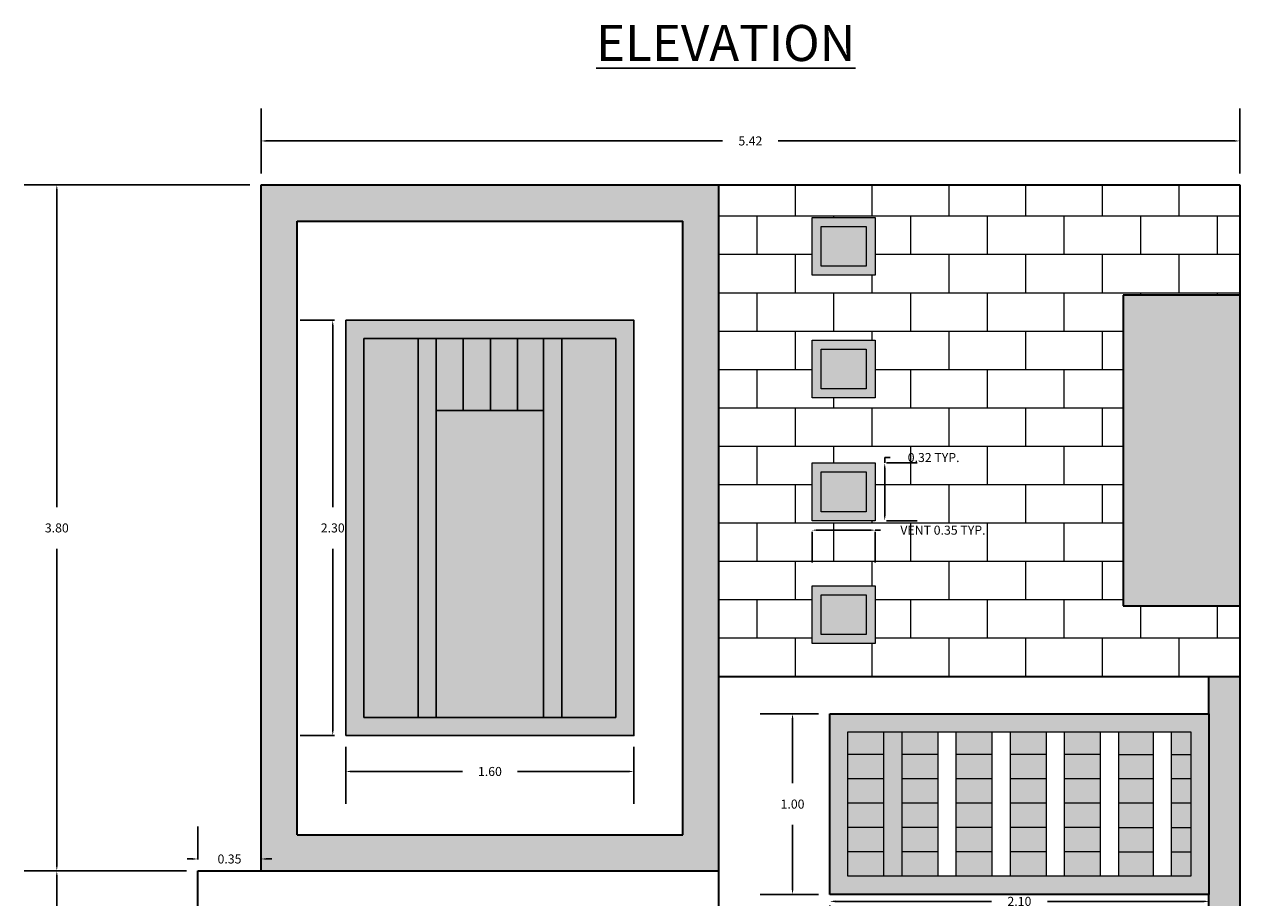
# Model space of a CAD drawing. Units: metres. Extents: x -184.63 to -177.08, y -586.84 to -578.06.
# Tile 2 of 2: x -183.87 to -177.14, y -582.9 to -578.06. Entities that reach past the tile are written whole.
import ezdxf

# ---------------------------------------------------------------- set-up
doc = ezdxf.new("R2010")
doc.units = ezdxf.units.M
doc.header["$MEASUREMENT"] = 0
for name, color, linetype, lineweight in [('A-ANNO-DIMS', 2, 'Continuous', 18), ('A-ANNO-TEXT', 7, 'Continuous', 25), ('A-DOOR', 4, 'Continuous', 25), ('A-ELEV', 7, 'Continuous', 35), ('A-ELEV-PATT', 8, 'Continuous', 13), ('A-GLAZ', 3, 'Continuous', 18)]:
    doc.layers.add(name, color=color, linetype=linetype, lineweight=lineweight)
doc.styles.get("Standard").update_dxf_attribs({"font": 'arial.ttf'})
doc.dimstyles.get("Standard").update_dxf_attribs({"dimtxt": 0.05, "dimasz": 0.03, "dimexe": 0.18, "dimexo": 0.0625, "dimgap": 0.09, "dimtad": 0, "dimtih": 1, "dimtoh": 1, "dimzin": 0, "dimdsep": 46, "dimtxsty": 'Standard', "dimcen": 0.09, "dimadec": 0, "dimazin": 0, "dimtfac": 1, "dimtofl": 0, "dimtmove": 0, "dimatfit": 3, "dimfxl": 1, "dimtolj": 1, "dimtzin": 0, "dimarcsym": 0})

# ---------------------------------------------------------------- blocks, each defined once
blk = doc.blocks.new('*D2')
at = {"layer": 'A-ANNO-DIMS', "color": 0, "lineweight": -2, "transparency": 16777216}
for p, q in [((-182.9705, -582.7541), (-183.8693, -582.7541)), ((-183.6893, -582.7841), (-183.6893, -583.844)), ((-183.6893, -585.1341), (-183.6893, -584.0742)), ((-183.2005, -585.1641), (-183.8693, -585.1641))]:
    blk.add_line(p, q, dxfattribs=at)
at = {"layer": 'A-ANNO-DIMS', "color": 0, "transparency": 16777216}
for points in [[(-183.6943, -582.7841), (-183.6843, -582.7841), (-183.6893, -582.7541)], [(-183.6943, -585.1341), (-183.6843, -585.1341), (-183.6893, -585.1641)]]:
    blk.add_solid(points, dxfattribs=at)
at = {"layer": 'Defpoints', "color": 0, "transparency": 16777216}
for p in [(-183.6893, -582.7541), (-182.908, -582.7541), (-183.138, -585.1641)]:
    blk.add_point(p, dxfattribs=at)
at = {"layer": 'A-ANNO-DIMS', "color": 0, "transparency": 16777216, "insert": (-183.6893, -583.9591), "char_height": 0.05, "attachment_point": 5}
blk.add_mtext('\\A1;2.41', dxfattribs=at)
blk = doc.blocks.new('*D3')
at = {"layer": 'A-ANNO-DIMS', "color": 0, "lineweight": -2, "transparency": 16777216}
for p, q in [((-182.6205, -578.9541), (-183.8693, -578.9541)), ((-183.6893, -578.9841), (-183.6893, -580.7386)), ((-183.6893, -582.7241), (-183.6893, -580.9697)), ((-182.9705, -582.7541), (-183.8693, -582.7541))]:
    blk.add_line(p, q, dxfattribs=at)
at = {"layer": 'A-ANNO-DIMS', "color": 0, "transparency": 16777216}
for points in [[(-183.6943, -578.9841), (-183.6843, -578.9841), (-183.6893, -578.9541)], [(-183.6943, -582.7241), (-183.6843, -582.7241), (-183.6893, -582.7541)]]:
    blk.add_solid(points, dxfattribs=at)
at = {"layer": 'Defpoints', "color": 0, "transparency": 16777216}
for p in [(-183.6893, -578.9541), (-182.558, -578.9541), (-182.908, -582.7541)]:
    blk.add_point(p, dxfattribs=at)
at = {"layer": 'A-ANNO-DIMS', "color": 0, "transparency": 16777216, "insert": (-183.6893, -580.8541), "char_height": 0.05, "attachment_point": 5}
blk.add_mtext('\\A1;3.80', dxfattribs=at)
blk = doc.blocks.new('*D9')
at = {"layer": 'A-ANNO-DIMS', "color": 0, "lineweight": -2, "transparency": 16777216}
for p, q in [((-182.908, -582.6916), (-182.908, -582.508)), ((-182.558, -582.6916), (-182.558, -582.508)), ((-182.938, -582.688), (-182.968, -582.688)), ((-182.528, -582.688), (-182.498, -582.688))]:
    blk.add_line(p, q, dxfattribs=at)
at = {"layer": 'A-ANNO-DIMS', "color": 0, "transparency": 16777216}
for points in [[(-182.938, -582.683), (-182.938, -582.693), (-182.908, -582.688)], [(-182.528, -582.683), (-182.528, -582.693), (-182.558, -582.688)]]:
    blk.add_solid(points, dxfattribs=at)
at = {"layer": 'Defpoints', "color": 0, "transparency": 16777216}
for p in [(-182.558, -582.688), (-182.908, -582.7541), (-182.558, -582.7541)]:
    blk.add_point(p, dxfattribs=at)
at = {"layer": 'A-ANNO-DIMS', "color": 0, "transparency": 16777216, "insert": (-182.733, -582.688), "char_height": 0.05, "attachment_point": 5}
blk.add_mtext('\\A1;0.35', dxfattribs=at)
blk = doc.blocks.new('*D10')
at = {"layer": 'A-ANNO-DIMS', "color": 0, "lineweight": -2, "transparency": 16777216}
for p, q in [((-182.088, -582.0666), (-182.088, -582.3832)), ((-180.493, -582.0666), (-180.493, -582.3832)), ((-182.058, -582.2032), (-181.443, -582.2032)), ((-180.523, -582.2032), (-181.138, -582.2032))]:
    blk.add_line(p, q, dxfattribs=at)
at = {"layer": 'A-ANNO-DIMS', "color": 0, "transparency": 16777216}
for points in [[(-182.058, -582.1982), (-182.058, -582.2082), (-182.088, -582.2032)], [(-180.523, -582.1982), (-180.523, -582.2082), (-180.493, -582.2032)]]:
    blk.add_solid(points, dxfattribs=at)
at = {"layer": 'Defpoints', "color": 0, "transparency": 16777216}
for p in [(-182.088, -582.0041), (-180.493, -582.0041), (-180.493, -582.2032)]:
    blk.add_point(p, dxfattribs=at)
at = {"layer": 'A-ANNO-DIMS', "color": 0, "transparency": 16777216, "insert": (-181.2905, -582.2032), "char_height": 0.05, "attachment_point": 5}
blk.add_mtext('\\A1;1.60', dxfattribs=at)
blk = doc.blocks.new('*D11')
at = {"layer": 'A-ANNO-DIMS', "color": 0, "lineweight": -2, "transparency": 16777216}
for p, q in [((-182.1505, -579.7041), (-182.3411, -579.7041)), ((-182.1611, -579.7341), (-182.1611, -580.7386)), ((-182.1611, -581.9741), (-182.1611, -580.9697)), ((-182.1505, -582.0041), (-182.3411, -582.0041))]:
    blk.add_line(p, q, dxfattribs=at)
at = {"layer": 'A-ANNO-DIMS', "color": 0, "transparency": 16777216}
for points in [[(-182.1661, -579.7341), (-182.1561, -579.7341), (-182.1611, -579.7041)], [(-182.1661, -581.9741), (-182.1561, -581.9741), (-182.1611, -582.0041)]]:
    blk.add_solid(points, dxfattribs=at)
at = {"layer": 'Defpoints', "color": 0, "transparency": 16777216}
for p in [(-182.088, -579.7041), (-182.1611, -582.0041), (-182.088, -582.0041)]:
    blk.add_point(p, dxfattribs=at)
at = {"layer": 'A-ANNO-DIMS', "color": 0, "transparency": 16777216, "insert": (-182.1611, -580.8541), "char_height": 0.05, "attachment_point": 5}
blk.add_mtext('\\A1;2.30', dxfattribs=at)
blk = doc.blocks.new('*D13')
at = {"layer": 'A-ANNO-DIMS', "color": 0, "lineweight": -2, "transparency": 16777216}
for p, q in [((-179.4705, -581.884), (-179.7945, -581.884)), ((-179.6145, -581.914), (-179.6145, -582.2685)), ((-179.6145, -582.854), (-179.6145, -582.4995)), ((-179.4705, -582.884), (-179.7945, -582.884))]:
    blk.add_line(p, q, dxfattribs=at)
at = {"layer": 'A-ANNO-DIMS', "color": 0, "transparency": 16777216}
for points in [[(-179.6195, -581.914), (-179.6095, -581.914), (-179.6145, -581.884)], [(-179.6195, -582.854), (-179.6095, -582.854), (-179.6145, -582.884)]]:
    blk.add_solid(points, dxfattribs=at)
at = {"layer": 'Defpoints', "color": 0, "transparency": 16777216}
for p in [(-179.408, -581.884), (-179.6145, -582.884), (-179.408, -582.884)]:
    blk.add_point(p, dxfattribs=at)
at = {"layer": 'A-ANNO-DIMS', "color": 0, "transparency": 16777216, "insert": (-179.6145, -582.384), "char_height": 0.05, "attachment_point": 5}
blk.add_mtext('\\A1;1.00', dxfattribs=at)
blk = doc.blocks.new('*D14')
at = {"layer": 'A-ANNO-DIMS', "color": 0, "lineweight": -2, "transparency": 16777216}
for p, q in [((-179.378, -582.9228), (-178.5133, -582.9228)), ((-177.338, -582.9228), (-178.2027, -582.9228)), ((-179.408, -582.9465), (-179.408, -583.1028)), ((-177.308, -582.9465), (-177.308, -583.1028))]:
    blk.add_line(p, q, dxfattribs=at)
at = {"layer": 'A-ANNO-DIMS', "color": 0, "transparency": 16777216}
for points in [[(-179.378, -582.9178), (-179.378, -582.9278), (-179.408, -582.9228)], [(-177.338, -582.9178), (-177.338, -582.9278), (-177.308, -582.9228)]]:
    blk.add_solid(points, dxfattribs=at)
at = {"layer": 'Defpoints', "color": 0, "transparency": 16777216}
for p in [(-179.408, -582.884), (-177.308, -582.884), (-177.308, -582.9228)]:
    blk.add_point(p, dxfattribs=at)
at = {"layer": 'A-ANNO-DIMS', "color": 0, "transparency": 16777216, "insert": (-178.358, -582.9228), "char_height": 0.05, "attachment_point": 5}
blk.add_mtext('\\A1;2.10', dxfattribs=at)
blk = doc.blocks.new('*D18')
at = {"layer": 'A-ANNO-DIMS', "color": 0, "lineweight": -2, "transparency": 16777216}
for p, q in [((-182.558, -578.8916), (-182.558, -578.5305)), ((-177.138, -578.8916), (-177.138, -578.5305)), ((-182.528, -578.7105), (-180.0027, -578.7105)), ((-177.168, -578.7105), (-179.6933, -578.7105))]:
    blk.add_line(p, q, dxfattribs=at)
at = {"layer": 'A-ANNO-DIMS', "color": 0, "transparency": 16777216}
for points in [[(-182.528, -578.7055), (-182.528, -578.7155), (-182.558, -578.7105)], [(-177.168, -578.7055), (-177.168, -578.7155), (-177.138, -578.7105)]]:
    blk.add_solid(points, dxfattribs=at)
at = {"layer": 'Defpoints', "color": 0, "transparency": 16777216}
for p in [(-177.138, -578.7105), (-182.558, -578.9541), (-177.138, -578.9541)]:
    blk.add_point(p, dxfattribs=at)
at = {"layer": 'A-ANNO-DIMS', "color": 0, "transparency": 16777216, "insert": (-179.848, -578.7105), "char_height": 0.05, "attachment_point": 5}
blk.add_mtext('\\A1;5.42', dxfattribs=at)
blk = doc.blocks.new('VENT')
for points in [[(-179.5065, -580.4941), (-179.1565, -580.4941), (-179.1565, -580.8141), (-179.5065, -580.8141)], [(-179.4565, -580.5441), (-179.2065, -580.5441), (-179.2065, -580.7641), (-179.4565, -580.7641)]]:
    blk.add_lwpolyline(points, close=True)
blk = doc.blocks.new('*D20')
at = {"layer": 'A-ANNO-DIMS', "color": 0, "lineweight": -2, "transparency": 16777216}
for p, q in [((-179.5065, -580.8766), (-179.5065, -581.0466)), ((-179.4765, -580.8666), (-179.1865, -580.8666)), ((-179.1565, -580.8666), (-179.1265, -580.8666)), ((-179.1565, -580.8766), (-179.1565, -581.0466))]:
    blk.add_line(p, q, dxfattribs=at)
at = {"layer": 'A-ANNO-DIMS', "color": 0, "transparency": 16777216}
for points in [[(-179.4765, -580.8616), (-179.4765, -580.8716), (-179.5065, -580.8666)], [(-179.1865, -580.8616), (-179.1865, -580.8716), (-179.1565, -580.8666)]]:
    blk.add_solid(points, dxfattribs=at)
at = {"layer": 'Defpoints', "color": 0, "transparency": 16777216}
for p in [(-179.5065, -580.8141), (-179.1565, -580.8141), (-179.1565, -580.8666)]:
    blk.add_point(p, dxfattribs=at)
at = {"layer": 'A-ANNO-DIMS', "color": 0, "transparency": 16777216, "insert": (-178.7815, -580.8666), "char_height": 0.05, "attachment_point": 5}
blk.add_mtext('\\A1;VENT 0.35 TYP.', dxfattribs=at)
blk = doc.blocks.new('*D21')
at = {"layer": 'A-ANNO-DIMS', "color": 0, "lineweight": -2, "transparency": 16777216}
for p, q in [((-179.104, -580.4941), (-179.104, -580.4641)), ((-179.104, -580.4641), (-179.074, -580.4641)), ((-179.094, -580.4941), (-178.924, -580.4941)), ((-179.104, -580.7841), (-179.104, -580.5241)), ((-179.094, -580.8141), (-178.924, -580.8141))]:
    blk.add_line(p, q, dxfattribs=at)
at = {"layer": 'A-ANNO-DIMS', "color": 0, "transparency": 16777216}
for points in [[(-179.109, -580.5241), (-179.099, -580.5241), (-179.104, -580.4941)], [(-179.109, -580.7841), (-179.099, -580.7841), (-179.104, -580.8141)]]:
    blk.add_solid(points, dxfattribs=at)
at = {"layer": 'Defpoints', "color": 0, "transparency": 16777216}
for p in [(-179.1565, -580.4941), (-179.104, -580.4941), (-179.1565, -580.8141)]:
    blk.add_point(p, dxfattribs=at)
at = {"layer": 'A-ANNO-DIMS', "color": 0, "transparency": 16777216, "insert": (-178.8331, -580.4641), "char_height": 0.05, "attachment_point": 5}
blk.add_mtext('\\A1;0.32 TYP.', dxfattribs=at)

msp = doc.modelspace()

# ---------------------------------------------------------------- hatches: boundary and pattern name
at = {"layer": 'A-ELEV-PATT'}
h = msp.add_hatch(color=256, dxfattribs=at)
h.dxf.hatch_style = 1
h.set_gradient(color1=(0, 255, 255), color2=(16, 86, 137), name='INVSPHERICAL')
h.paths.add_polyline_path([(-180.023, -578.9541), (-182.558, -578.9541), (-182.558, -582.7541), (-180.023, -582.7541)])
h.paths.add_polyline_path([(-182.358, -582.5541), (-182.358, -579.1541), (-180.223, -579.1541), (-180.223, -582.5541)], flags=16)
h.paths.add_polyline_path([(-182.088, -582.0041), (-182.088, -579.7041), (-180.493, -579.7041), (-180.493, -582.0041), (-180.593, -582.0041)], flags=0)
h.paths.add_polyline_path([(-181.988, -581.9041), (-181.988, -579.8041), (-180.593, -579.8041), (-180.593, -581.9041)], flags=0)
h = msp.add_hatch(dxfattribs=at)
h.set_pattern_fill('BRICK', color=256, scale=0.85)
h.set_pattern_definition([(0, (-180.023, -581.67628), (0, 0.2125), []), (90, (-180.023, -581.6763), (-0.425, 0), [0.2125, -0.2125]), (90, (-179.8105, -581.6763), (-0.425, 0), [-0.2125, 0.2125])])
h.paths.add_polyline_path([(-177.7834, -579.5645), (-177.138, -579.5645), (-177.138, -578.9541), (-180.023, -578.9541), (-180.023, -581.6763), (-177.138, -581.6763), (-177.138, -581.2856), (-177.7834, -581.2856)])
h.paths.add_polyline_path([(-179.1565, -580.8141), (-179.5065, -580.8141), (-179.5065, -580.4941), (-179.1565, -580.4941)], flags=16)
h.paths.add_polyline_path([(-179.1565, -581.1752), (-179.1565, -581.4952), (-179.5065, -581.4952), (-179.5065, -581.1752)], flags=16)
h.paths.add_polyline_path([(-179.2065, -580.7641), (-179.4565, -580.7641), (-179.4565, -580.5441), (-179.2065, -580.5441)], flags=0)
h.paths.add_polyline_path([(-179.2065, -581.2252), (-179.2065, -581.4452), (-179.4565, -581.4452), (-179.4565, -581.2252)], flags=0)
h.paths.add_polyline_path([(-179.1565, -580.1341), (-179.5065, -580.1341), (-179.5065, -579.8141), (-179.1565, -579.8141)], flags=16)
h.paths.add_polyline_path([(-179.2065, -580.0841), (-179.4565, -580.0841), (-179.4565, -579.8641), (-179.2065, -579.8641)], flags=0)
h.paths.add_polyline_path([(-179.1565, -579.4541), (-179.5065, -579.4541), (-179.5065, -579.1341), (-179.1565, -579.1341)], flags=16)
h.paths.add_polyline_path([(-179.2065, -579.4041), (-179.4565, -579.4041), (-179.4565, -579.1841), (-179.2065, -579.1841)], flags=0)
h = msp.add_hatch(color=256, dxfattribs=at)
h.dxf.hatch_style = 1
h.set_gradient(color1=(0, 255, 255), color2=(16, 86, 137), name='INVCYLINDER')
h.paths.add_polyline_path([(-179.1565, -579.1341), (-179.5065, -579.1341), (-179.5065, -579.4541), (-179.1565, -579.4541)])
h.paths.add_polyline_path([(-179.2065, -579.1841), (-179.2065, -579.4041), (-179.4565, -579.4041), (-179.4565, -579.1841)], flags=16)
h.paths.add_polyline_path([(-179.1565, -579.8141), (-179.5065, -579.8141), (-179.5065, -580.1341), (-179.1565, -580.1341)])
h.paths.add_polyline_path([(-179.2065, -580.0841), (-179.4565, -580.0841), (-179.4565, -579.8641), (-179.2065, -579.8641)], flags=16)
h.paths.add_polyline_path([(-179.1565, -580.4941), (-179.5065, -580.4941), (-179.5065, -580.8141), (-179.1565, -580.8141)])
h.paths.add_polyline_path([(-179.2065, -580.5441), (-179.2065, -580.7641), (-179.4565, -580.7641), (-179.4565, -580.5441)], flags=16)
h.paths.add_polyline_path([(-179.1565, -581.1752), (-179.5065, -581.1752), (-179.5065, -581.4952), (-179.1565, -581.4952)])
h.paths.add_polyline_path([(-179.2065, -581.2252), (-179.2065, -581.4452), (-179.4565, -581.4452), (-179.4565, -581.2252)], flags=16)
h = msp.add_hatch(color=256, dxfattribs=at)
h.dxf.hatch_style = 1
h.set_gradient(color1=(0, 255, 255), color2=(173, 221, 247))
h.paths.add_polyline_path([(-179.2065, -579.1841), (-179.4565, -579.1841), (-179.4565, -579.4041), (-179.2065, -579.4041)])
h.paths.add_polyline_path([(-179.2065, -579.8641), (-179.4565, -579.8641), (-179.4565, -580.0841), (-179.2065, -580.0841)])
h.paths.add_polyline_path([(-179.2065, -580.5441), (-179.4565, -580.5441), (-179.4565, -580.7641), (-179.2065, -580.7641)])
h.paths.add_polyline_path([(-179.2065, -581.2252), (-179.4565, -581.2252), (-179.4565, -581.4452), (-179.2065, -581.4452)])
h = msp.add_hatch(color=256, dxfattribs=at)
h.dxf.hatch_style = 1
h.set_gradient(color1=(0, 255, 255), color2=(0, 0, 255), name='INVCURVED')
h.paths.add_polyline_path([(-177.138, -579.5645), (-177.7834, -579.5645), (-177.7834, -581.2856), (-177.138, -581.2856)])
h = msp.add_hatch(color=256, dxfattribs=at)
h.dxf.hatch_style = 1
h.set_gradient(color1=(0, 0, 255), color2=(0, 255, 255), name='SPHERICAL')
h.paths.add_polyline_path([(-180.493, -579.7041), (-182.088, -579.7041), (-182.088, -582.0041), (-180.493, -582.0041)])
h.paths.add_polyline_path([(-180.593, -579.8041), (-180.593, -581.9041), (-181.988, -581.9041), (-181.988, -579.8041)], flags=16)
h.paths.add_polyline_path([(-181.688, -579.8041), (-181.988, -579.8041), (-181.988, -581.9041), (-181.688, -581.9041)], flags=0)
h.paths.add_polyline_path([(-180.993, -580.2041), (-181.588, -580.2041), (-181.588, -581.9041), (-180.993, -581.9041)], flags=0)
h.paths.add_polyline_path([(-180.593, -579.8041), (-180.893, -579.8041), (-180.893, -581.9041), (-180.593, -581.9041)], flags=0)
h.paths.add_polyline_path([(-180.893, -579.8041), (-180.993, -579.8041), (-180.993, -581.9041), (-180.893, -581.9041)], flags=0)
h.paths.add_polyline_path([(-181.588, -580.2041), (-181.588, -579.8041), (-181.688, -579.8041), (-181.688, -581.9041), (-181.588, -581.9041)], flags=0)
h.paths.add_polyline_path([(-181.138, -579.8041), (-181.288, -579.8041), (-181.288, -580.2041), (-181.138, -580.2041)], flags=0)
h.paths.add_polyline_path([(-181.288, -579.8041), (-181.438, -579.8041), (-181.438, -580.2041), (-181.288, -580.2041)], flags=0)
h = msp.add_hatch(color=256, dxfattribs=at)
h.dxf.hatch_style = 1
h.set_gradient(color1=(0, 255, 255), color2=(16, 86, 137), name='INVSPHERICAL')
h.paths.add_polyline_path([(-180.993, -580.2041), (-181.588, -580.2041), (-181.588, -581.9041), (-180.993, -581.9041)])
h.paths.add_polyline_path([(-181.588, -580.2041), (-181.588, -579.8041), (-181.688, -579.8041), (-181.688, -581.9041), (-181.588, -581.9041)])
h.paths.add_polyline_path([(-181.688, -579.8041), (-181.988, -579.8041), (-181.988, -581.9041), (-181.688, -581.9041)])
h.paths.add_polyline_path([(-180.593, -579.8041), (-180.893, -579.8041), (-180.893, -581.9041), (-180.593, -581.9041)])
h.paths.add_polyline_path([(-180.893, -579.8041), (-180.993, -579.8041), (-180.993, -581.9041), (-180.893, -581.9041)])
h.paths.add_polyline_path([(-181.438, -579.8041), (-181.588, -579.8041), (-181.588, -580.2041), (-181.438, -580.2041)])
h.paths.add_polyline_path([(-181.288, -579.8041), (-181.438, -579.8041), (-181.438, -580.2041), (-181.288, -580.2041)])
h.paths.add_polyline_path([(-180.993, -579.8041), (-181.138, -579.8041), (-181.138, -580.2041), (-180.993, -580.2041)])
h.paths.add_polyline_path([(-181.138, -579.8041), (-181.288, -579.8041), (-181.288, -580.2041), (-181.138, -580.2041)])
h.paths.add_polyline_path([(-180.768, -583.0941), (-181.068, -583.0941), (-181.068, -584.8241), (-180.768, -584.8241)])
h.paths.add_polyline_path([(-181.068, -583.0941), (-181.168, -583.0941), (-181.168, -584.8241), (-181.068, -584.8241)])
h.paths.add_polyline_path([(-181.863, -583.0941), (-182.163, -583.0941), (-182.163, -584.8241), (-181.863, -584.8241)])
h.paths.add_polyline_path([(-181.763, -583.0941), (-181.863, -583.0941), (-181.863, -584.8241), (-181.763, -584.8241)])
h.paths.add_polyline_path([(-181.168, -583.4941), (-181.763, -583.4941), (-181.763, -584.8241), (-181.168, -584.8241)])
h.paths.add_polyline_path([(-181.613, -583.0941), (-181.763, -583.0941), (-181.763, -583.4941), (-181.613, -583.4941)])
h.paths.add_polyline_path([(-181.463, -583.0941), (-181.613, -583.0941), (-181.613, -583.4941), (-181.463, -583.4941)])
h.paths.add_polyline_path([(-181.313, -583.0941), (-181.463, -583.0941), (-181.463, -583.4941), (-181.313, -583.4941)])
h.paths.add_polyline_path([(-181.168, -583.0941), (-181.313, -583.0941), (-181.313, -583.4941), (-181.168, -583.4941)])
h.paths.add_polyline_path([(-178.6925, -583.6277), (-179.2875, -583.6277), (-179.2875, -584.9577), (-178.6925, -584.9577)])
h.paths.add_polyline_path([(-179.3875, -583.2277), (-179.6875, -583.2277), (-179.6875, -584.9577), (-179.3875, -584.9577)])
h.paths.add_polyline_path([(-179.2875, -583.6277), (-179.2875, -583.2277), (-179.3875, -583.2277), (-179.3875, -584.9577), (-179.2875, -584.9577)])
h.paths.add_polyline_path([(-179.1375, -583.2277), (-179.2875, -583.2277), (-179.2875, -583.6277), (-179.1375, -583.6277)])
h.paths.add_polyline_path([(-178.9875, -583.2277), (-179.1375, -583.2277), (-179.1375, -583.6277), (-178.9875, -583.6277)])
h.paths.add_polyline_path([(-178.8375, -583.2277), (-178.9875, -583.2277), (-178.9875, -583.6277), (-178.8375, -583.6277)])
h.paths.add_polyline_path([(-178.5925, -583.2277), (-178.6925, -583.2277), (-178.6925, -584.9577), (-178.5925, -584.9577)])
h.paths.add_polyline_path([(-178.6925, -583.2277), (-178.8375, -583.2277), (-178.8375, -583.6277), (-178.6925, -583.6277)])
h.paths.add_polyline_path([(-178.2925, -583.2277), (-178.5925, -583.2277), (-178.5925, -584.9577), (-178.2925, -584.9577)])
h = msp.add_hatch(color=256, dxfattribs=at)
h.dxf.hatch_style = 1
h.paths.add_polyline_path([(-177.138, -581.6763), (-177.308, -581.6763), (-177.308, -581.884), (-177.308, -582.884), (-177.308, -585.8641), (-177.138, -585.8641), (-177.138, -585.1641)])
h = msp.add_hatch(color=256, dxfattribs=at)
h.dxf.hatch_style = 1
h.set_gradient(color1=(0, 0, 255), color2=(0, 255, 255), name='SPHERICAL')
h.paths.add_polyline_path([(-180.668, -582.9941), (-182.263, -582.9941), (-182.263, -584.9241), (-180.668, -584.9241)])
h.paths.add_polyline_path([(-182.163, -583.0941), (-180.768, -583.0941), (-180.768, -584.8241), (-182.163, -584.8241)], flags=16)
h.paths.add_polyline_path([(-178.1925, -583.1277), (-179.7875, -583.1277), (-179.7875, -585.0577), (-178.1925, -585.0577)])
h.paths.add_polyline_path([(-178.2925, -583.2277), (-178.2925, -584.9577), (-179.6875, -584.9577), (-179.6875, -583.2277)], flags=16)
h.paths.add_polyline_path([(-177.308, -581.884), (-179.408, -581.884), (-179.408, -582.884), (-177.308, -582.884)])
h.paths.add_polyline_path([(-177.408, -581.984), (-177.408, -582.784), (-179.308, -582.784), (-179.308, -581.984)], flags=16)
h = msp.add_hatch(color=256, dxfattribs=at)
h.dxf.hatch_style = 1
h.set_gradient(color1=(0, 255, 255), color2=(16, 86, 137), name='SPHERICAL')
h.paths.add_polyline_path([(-179.108, -581.984), (-179.308, -581.984), (-179.308, -582.1097), (-179.108, -582.1097)])
h.paths.add_polyline_path([(-179.108, -582.1097), (-179.308, -582.1097), (-179.308, -582.2445), (-179.108, -582.2445)])
h.paths.add_polyline_path([(-179.108, -582.2445), (-179.308, -582.2445), (-179.308, -582.3794), (-179.108, -582.3794)])
h.paths.add_polyline_path([(-179.108, -582.3794), (-179.308, -582.3794), (-179.308, -582.5143), (-179.108, -582.5143)])
h.paths.add_polyline_path([(-179.108, -582.5143), (-179.308, -582.5143), (-179.308, -582.6491), (-179.108, -582.6491)])
h.paths.add_polyline_path([(-179.108, -582.6491), (-179.308, -582.6491), (-179.308, -582.784), (-179.108, -582.784)])
h.paths.add_polyline_path([(-178.808, -582.6491), (-179.008, -582.6491), (-179.008, -582.784), (-178.808, -582.784)])
h.paths.add_polyline_path([(-178.808, -582.5143), (-179.008, -582.5143), (-179.008, -582.6491), (-178.808, -582.6491)])
h.paths.add_polyline_path([(-178.808, -582.3794), (-179.008, -582.3794), (-179.008, -582.5143), (-178.808, -582.5143)])
h.paths.add_polyline_path([(-178.808, -582.2445), (-179.008, -582.2445), (-179.008, -582.3794), (-178.808, -582.3794)])
h.paths.add_polyline_path([(-178.808, -582.1097), (-179.008, -582.1097), (-179.008, -582.2445), (-178.808, -582.2445)])
h.paths.add_polyline_path([(-178.808, -581.984), (-179.008, -581.984), (-179.008, -582.1097), (-178.808, -582.1097)])
h.paths.add_polyline_path([(-178.508, -581.984), (-178.708, -581.984), (-178.708, -582.1097), (-178.508, -582.1097)])
h.paths.add_polyline_path([(-178.508, -582.6491), (-178.708, -582.6491), (-178.708, -582.784), (-178.508, -582.784)])
h.paths.add_polyline_path([(-178.508, -582.5143), (-178.708, -582.5143), (-178.708, -582.6491), (-178.508, -582.6491)])
h.paths.add_polyline_path([(-178.508, -582.3794), (-178.708, -582.3794), (-178.708, -582.5143), (-178.508, -582.5143)])
h.paths.add_polyline_path([(-178.508, -582.2445), (-178.708, -582.2445), (-178.708, -582.3794), (-178.508, -582.3794)])
h.paths.add_polyline_path([(-178.508, -582.1097), (-178.708, -582.1097), (-178.708, -582.2445), (-178.508, -582.2445)])
h.paths.add_polyline_path([(-178.208, -581.984), (-178.408, -581.984), (-178.408, -582.1097), (-178.208, -582.1097)])
h.paths.add_polyline_path([(-178.208, -582.1097), (-178.408, -582.1097), (-178.408, -582.2445), (-178.208, -582.2445)])
h.paths.add_polyline_path([(-178.208, -582.2445), (-178.408, -582.2445), (-178.408, -582.3794), (-178.208, -582.3794)])
h.paths.add_polyline_path([(-178.208, -582.3794), (-178.408, -582.3794), (-178.408, -582.5143), (-178.208, -582.5143)])
h.paths.add_polyline_path([(-178.208, -582.6491), (-178.408, -582.6491), (-178.408, -582.784), (-178.208, -582.784)])
h.paths.add_polyline_path([(-178.208, -582.5143), (-178.408, -582.5143), (-178.408, -582.6491), (-178.208, -582.6491)])
h.paths.add_polyline_path([(-177.908, -581.984), (-178.108, -581.984), (-178.108, -582.1097), (-177.908, -582.1097)])
h.paths.add_polyline_path([(-177.908, -582.1097), (-178.108, -582.1097), (-178.108, -582.2445), (-177.908, -582.2445)])
h.paths.add_polyline_path([(-177.908, -582.2445), (-178.108, -582.2445), (-178.108, -582.3794), (-177.908, -582.3794)])
h.paths.add_polyline_path([(-177.908, -582.3794), (-178.108, -582.3794), (-178.108, -582.5143), (-177.908, -582.5143)])
h.paths.add_polyline_path([(-177.908, -582.5143), (-178.108, -582.5143), (-178.108, -582.6491), (-177.908, -582.6491)])
h.paths.add_polyline_path([(-177.908, -582.6491), (-178.108, -582.6491), (-178.108, -582.784), (-177.908, -582.784)])
h.paths.add_polyline_path([(-177.6162, -581.984), (-177.808, -581.984), (-177.808, -582.1097), (-177.6162, -582.1097)])
h.paths.add_polyline_path([(-177.6162, -582.1097), (-177.808, -582.1097), (-177.808, -582.2427), (-177.6162, -582.2427)])
h.paths.add_polyline_path([(-177.6162, -582.2427), (-177.808, -582.2427), (-177.808, -582.3776), (-177.6162, -582.3776)])
h.paths.add_polyline_path([(-177.6162, -582.3776), (-177.808, -582.3776), (-177.808, -582.514), (-177.6162, -582.514)])
h.paths.add_polyline_path([(-177.6162, -582.514), (-177.808, -582.514), (-177.808, -582.6489), (-177.6162, -582.6489)])
h.paths.add_polyline_path([(-177.6162, -582.6489), (-177.808, -582.6489), (-177.808, -582.784), (-177.6162, -582.784)])
h.paths.add_polyline_path([(-177.408, -581.984), (-177.5162, -581.984), (-177.5162, -582.1097), (-177.408, -582.1097)])
h.paths.add_polyline_path([(-177.408, -582.1097), (-177.5162, -582.1097), (-177.5162, -582.2427), (-177.408, -582.2427)])
h.paths.add_polyline_path([(-177.408, -582.2427), (-177.5162, -582.2427), (-177.5162, -582.3776), (-177.408, -582.3776)])
h.paths.add_polyline_path([(-177.408, -582.3776), (-177.5162, -582.3776), (-177.5162, -582.514), (-177.408, -582.514)])
h.paths.add_polyline_path([(-177.408, -582.514), (-177.5162, -582.514), (-177.5162, -582.6489), (-177.408, -582.6489)])
h.paths.add_polyline_path([(-177.408, -582.6489), (-177.5162, -582.6489), (-177.5162, -582.784), (-177.408, -582.784)])
h = msp.add_hatch(color=256, dxfattribs=at)
h.dxf.hatch_style = 1
h.set_gradient(color1=(0, 255, 255), color2=(16, 86, 137), name='INVSPHERICAL')
h.paths.add_polyline_path([(-179.008, -581.984), (-179.108, -581.984), (-179.108, -582.784), (-179.008, -582.784)])

# ---------------------------------------------------------------- linework, layer by layer
at = {"layer": 'A-DOOR'}
for p, q in [((-180.593, -579.8041), (-181.988, -579.8041)), ((-181.988, -579.8041), (-181.988, -581.9041)), ((-181.688, -579.8041), (-181.688, -581.9041)), ((-181.588, -579.8041), (-181.588, -581.9041)), ((-181.438, -579.8041), (-181.438, -580.2041)), ((-181.288, -579.8041), (-181.288, -580.2041)), ((-181.138, -579.8041), (-181.138, -580.2041)), ((-180.993, -581.9041), (-180.993, -579.8041)), ((-180.893, -581.9041), (-180.893, -579.8041)), ((-180.593, -581.9041), (-180.593, -579.8041)), ((-180.993, -580.2041), (-181.588, -580.2041)), ((-181.988, -581.9041), (-180.593, -581.9041)), ((-180.593, -582.0041), (-180.493, -582.0041))]:
    msp.add_line(p, q, dxfattribs=at)
msp.add_lwpolyline([(-182.088, -582.0041), (-180.493, -582.0041), (-180.493, -579.7041), (-182.088, -579.7041)], close=True, dxfattribs=at)
at = {"layer": 'A-ELEV'}
for p, q in [((-182.558, -582.7541), (-182.558, -578.9541)), ((-182.558, -578.9541), (-177.138, -578.9541)), ((-180.023, -585.1641), (-180.023, -578.9541)), ((-177.138, -578.9541), (-177.138, -585.1641)), ((-182.358, -582.5541), (-182.358, -579.1541)), ((-182.358, -579.1541), (-180.223, -579.1541)), ((-180.223, -582.5541), (-180.223, -579.1541)), ((-177.138, -579.5645), (-177.7834, -579.5645)), ((-177.7834, -579.5645), (-177.7834, -581.2856)), ((-177.7834, -581.2856), (-177.138, -581.2856)), ((-180.023, -581.6763), (-177.138, -581.6763)), ((-177.308, -581.884), (-177.308, -581.6763)), ((-179.408, -582.884), (-179.408, -581.884)), ((-179.408, -581.884), (-177.308, -581.884)), ((-177.308, -581.884), (-177.308, -582.884)), ((-182.358, -582.5541), (-180.223, -582.5541)), ((-182.908, -585.1641), (-182.908, -582.7541)), ((-182.908, -582.7541), (-182.558, -582.7541)), ((-182.558, -582.7541), (-180.023, -582.7541)), ((-177.308, -582.884), (-179.408, -582.884)), ((-179.408, -582.884), (-179.408, -582.884)), ((-177.308, -585.8641), (-177.308, -582.884))]:
    msp.add_line(p, q, dxfattribs=at)
at = {"layer": 'A-GLAZ'}
for p, q in [((-179.308, -581.984), (-177.408, -581.984)), ((-179.308, -582.784), (-179.308, -581.984)), ((-179.108, -582.784), (-179.108, -581.984)), ((-179.008, -582.784), (-179.008, -581.984)), ((-178.808, -582.784), (-178.808, -581.984)), ((-178.808, -582.784), (-178.808, -581.984)), ((-178.808, -582.784), (-178.808, -581.984)), ((-178.808, -582.784), (-178.808, -581.984)), ((-178.708, -582.784), (-178.708, -581.984)), ((-178.708, -582.784), (-178.708, -581.984)), ((-178.708, -582.784), (-178.708, -581.984)), ((-178.708, -582.784), (-178.708, -581.984)), ((-178.508, -582.784), (-178.508, -581.984)), ((-178.508, -582.784), (-178.508, -581.984)), ((-178.408, -582.784), (-178.408, -581.984)), ((-178.408, -582.784), (-178.408, -581.984)), ((-178.208, -582.784), (-178.208, -581.984)), ((-178.208, -582.784), (-178.208, -581.984)), ((-178.108, -582.784), (-178.108, -581.984)), ((-178.108, -582.784), (-178.108, -581.984)), ((-177.908, -582.784), (-177.908, -581.984)), ((-177.908, -582.784), (-177.908, -581.984)), ((-177.808, -582.784), (-177.808, -581.984)), ((-177.808, -582.784), (-177.808, -581.984)), ((-177.6162, -582.784), (-177.6162, -581.984)), ((-177.6162, -582.784), (-177.6162, -581.984)), ((-177.5162, -582.784), (-177.5162, -581.984)), ((-177.5162, -582.784), (-177.5162, -581.984)), ((-177.408, -581.984), (-177.408, -582.784)), ((-179.108, -582.1097), (-179.308, -582.1097)), ((-179.108, -582.1097), (-179.108, -582.1097)), ((-178.808, -582.1097), (-179.008, -582.1097)), ((-178.808, -582.1097), (-179.008, -582.1097)), ((-178.808, -582.1097), (-179.008, -582.1097)), ((-178.508, -582.1097), (-178.708, -582.1097)), ((-178.508, -582.1097), (-178.708, -582.1097)), ((-178.208, -582.1097), (-178.408, -582.1097)), ((-177.908, -582.1097), (-178.108, -582.1097)), ((-177.808, -582.1097), (-177.6162, -582.1097)), ((-177.5162, -582.1097), (-177.408, -582.1097)), ((-179.108, -582.2445), (-179.308, -582.2445)), ((-178.808, -582.2445), (-179.008, -582.2445)), ((-178.808, -582.2445), (-179.008, -582.2445)), ((-178.808, -582.2445), (-179.008, -582.2445)), ((-178.508, -582.2445), (-178.708, -582.2445)), ((-178.508, -582.2445), (-178.708, -582.2445)), ((-178.208, -582.2445), (-178.408, -582.2445)), ((-177.908, -582.2445), (-178.108, -582.2445)), ((-177.808, -582.2427), (-177.6162, -582.2427)), ((-177.808, -582.2427), (-177.6162, -582.2427)), ((-177.5162, -582.2427), (-177.408, -582.2427)), ((-179.108, -582.3794), (-179.308, -582.3794)), ((-178.808, -582.3794), (-179.008, -582.3794)), ((-178.808, -582.3794), (-179.008, -582.3794)), ((-178.808, -582.3794), (-179.008, -582.3794)), ((-178.508, -582.3794), (-178.708, -582.3794)), ((-178.508, -582.3794), (-178.708, -582.3794)), ((-178.208, -582.3794), (-178.408, -582.3794)), ((-177.908, -582.3794), (-178.108, -582.3794)), ((-177.808, -582.3776), (-177.6162, -582.3776)), ((-177.5162, -582.3776), (-177.408, -582.3776)), ((-179.108, -582.5143), (-179.308, -582.5143)), ((-178.808, -582.5143), (-179.008, -582.5143)), ((-178.808, -582.5143), (-179.008, -582.5143)), ((-178.808, -582.5143), (-179.008, -582.5143)), ((-178.508, -582.5143), (-178.708, -582.5143)), ((-178.508, -582.5143), (-178.708, -582.5143)), ((-178.208, -582.5143), (-178.408, -582.5143)), ((-177.908, -582.5143), (-178.108, -582.5143)), ((-177.808, -582.514), (-177.6162, -582.514)), ((-177.5162, -582.514), (-177.408, -582.514)), ((-179.108, -582.6491), (-179.308, -582.6491)), ((-178.808, -582.6491), (-179.008, -582.6491)), ((-178.808, -582.6491), (-179.008, -582.6491)), ((-178.808, -582.6491), (-179.008, -582.6491)), ((-178.508, -582.6491), (-178.708, -582.6491)), ((-178.508, -582.6491), (-178.708, -582.6491)), ((-178.208, -582.6491), (-178.408, -582.6491)), ((-177.908, -582.6491), (-178.108, -582.6491)), ((-177.808, -582.6489), (-177.6162, -582.6489)), ((-177.5162, -582.6489), (-177.408, -582.6489)), ((-177.408, -582.784), (-179.308, -582.784)), ((-179.108, -582.784), (-179.308, -582.784))]:
    msp.add_line(p, q, dxfattribs=at)

# ---------------------------------------------------------------- block references
for p in [(0, 1.36), (0, 0.68), (0, 0), (0, -0.6811)]:
    msp.add_blockref('VENT', p, dxfattribs=at)

# ---------------------------------------------------------------- texts
at = {"layer": 'A-ANNO-TEXT', "insert": (-180.7022, -578.068), "char_height": 0.2, "attachment_point": 1}
msp.add_mtext_dynamic_manual_height_columns('{\\fArial|b1|i0|c0|p34;\\LELEVATION}', width=5.939433, gutter_width=1, heights=[0], dxfattribs=at)

# ---------------------------------------------------------------- dimensions: what is measured, and where the dimension line sits
at = {"layer": 'A-ANNO-DIMS'}
for base, p1, p2, picture, middle in [((-177.138, -578.7105), (-182.558, -578.9541), (-177.138, -578.9541), '*D18', (-179.848, -578.7105)), ((-180.4929953712, -582.203231238), (-182.0879953712, -582.0041223595), (-180.4929953712, -582.0041223595), '*D10', (-181.2904953712, -582.203231238)), ((-182.558, -582.688), (-182.908, -582.7541), (-182.558, -582.7541), '*D9', (-182.733, -582.688)), ((-177.308, -582.9228), (-179.408, -582.884), (-177.308, -582.884), '*D14', (-178.358, -582.9228))]:
    dim = msp.add_linear_dim(base=base, p1=p1, p2=p2, dimstyle='Standard', override={"dimclrd": 0, "dimclre": 0, "dimclrt": 0}, dxfattribs=at)
    dim.commit()
    dim.dimension.update_dxf_attribs({"geometry": picture, "text_midpoint": middle})
for base, p1, p2, override, picture, middle in [((-183.6893, -578.9541), (-182.908, -582.7541), (-182.558, -578.9541), {"dimclrd": 0, "dimclre": 0, "dimclrt": 0, "dimtmove": 1}, '*D3', (-183.6893, -580.8541)), ((-182.1611, -582.0041), (-182.088, -579.7041), (-182.088, -582.0041), {"dimclrd": 0, "dimclre": 0, "dimclrt": 0}, '*D11', (-182.1611, -580.8541)), ((-179.6145, -582.884), (-179.408, -581.884), (-179.408, -582.884), {"dimclrd": 0, "dimclre": 0, "dimclrt": 0}, '*D13', (-179.6145, -582.384)), ((-183.6893, -582.7541), (-183.138, -585.1641), (-182.908, -582.7541), {"dimclrd": 0, "dimclre": 0, "dimclrt": 0, "dimtmove": 1}, '*D2', (-183.6893, -583.9591))]:
    dim = msp.add_linear_dim(base=base, p1=p1, p2=p2, angle=90, dimstyle='Standard', override=override, dxfattribs=at)
    dim.commit()
    dim.dimension.update_dxf_attribs({"geometry": picture, "text_midpoint": middle})
dim = msp.add_linear_dim(base=(-179.104, -580.4941), p1=(-179.1565, -580.8141), p2=(-179.1565, -580.4941), angle=90, text='<> TYP.', dimstyle='Standard', override={"dimdec": 2, "dimlfac": 1, "dimrnd": 0, "dimzin": 0, "dimdsep": 46, "dimlunit": 2}, dxfattribs=at)
dim.commit()
dim.dimension.update_dxf_attribs({"geometry": '*D21', "text_midpoint": (-178.8331, -580.4641)})
dim = msp.add_linear_dim(base=(-179.1565, -580.8666), p1=(-179.5065, -580.8141), p2=(-179.1565, -580.8141), text='VENT <> TYP.', dimstyle='Standard', override={"dimdec": 2, "dimlfac": 1, "dimrnd": 0, "dimzin": 0, "dimdsep": 46, "dimlunit": 2}, dxfattribs=at)
dim.commit()
dim.dimension.update_dxf_attribs({"geometry": '*D20', "text_midpoint": (-178.7815, -580.8666)})

doc.saveas('drawing.dxf')
